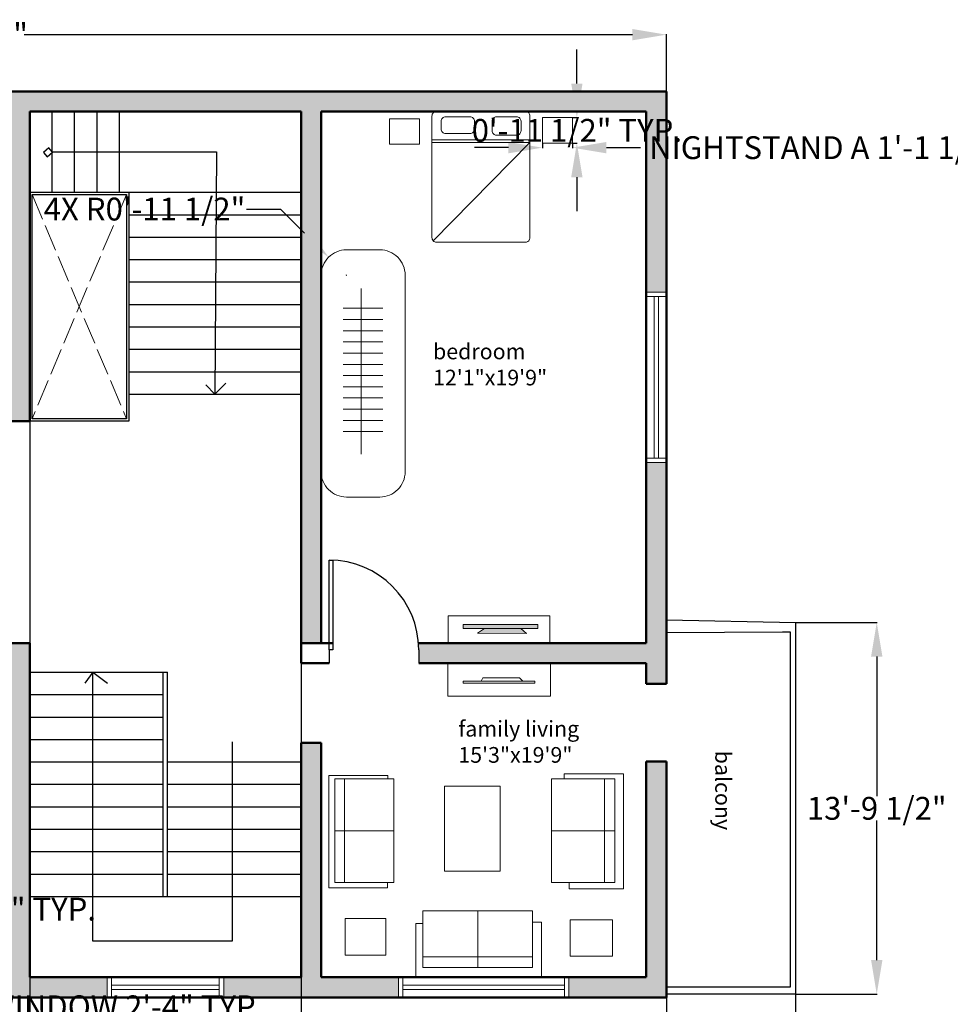
# Model space of a CAD drawing. Units: inches. Extents: x -2 to 7298, y -2 to 4583.
# Tile 5 of 6: x 6384 to 6799, y 4144 to 4583. Entities that reach past the tile are written whole.
import ezdxf

# ---------------------------------------------------------------- set-up
doc = ezdxf.new("R2010")
doc.units = ezdxf.units.IN
doc.header["$MEASUREMENT"] = 0
doc.linetypes.add('ACAD_ISO02W100', pattern=[15, 12, -3])
for name, color, linetype, lineweight in [('A-ANNO-DIMS', 2, 'Continuous', 18), ('A-AREA-IDEN', 7, 'Continuous', 18), ('A-DOOR', 4, 'Continuous', 25), ('A-FLOR-BALC', 7, 'Continuous', 25), ('A-FLOR-CASE', 30, 'Continuous', 18), ('A-FLOR-STRS', 7, 'Continuous', 25), ('A-FLOR-STRS-HIDN', 7, 'ACAD_ISO02W100', 18), ('A-FURN', 8, 'Continuous', 18), ('A-FURN-PATT', 18, 'Continuous', 13), ('A-GLAZ', 4, 'Continuous', 18), ('A-WALL', 7, 'Continuous', 50), ('A-WALL-PATT', 18, 'Continuous', 13)]:
    doc.layers.add(name, color=color, linetype=linetype, lineweight=lineweight)
doc.styles.get("Standard").update_dxf_attribs({"font": 'arial.ttf'})
doc.dimstyles.get("Standard").update_dxf_attribs({"dimtxt": 10.18, "dimasz": 15.18, "dimexe": 0.18, "dimexo": 0.0625, "dimgap": 0.09, "dimtad": 0, "dimtih": 1, "dimtoh": 1, "dimdec": 0, "dimzin": 0, "dimdsep": 46, "dimlunit": 3, "dimtxsty": 'Standard', "dimcen": 0.09, "dimadec": 0, "dimazin": 0, "dimtfac": 1, "dimtdec": 0, "dimtofl": 0, "dimtmove": 0, "dimatfit": 3, "dimfxl": 1, "dimtolj": 1, "dimtzin": 0, "dimarcsym": 0})

# ---------------------------------------------------------------- blocks, each defined once
blk = doc.blocks.new('*U2')
for p, q in [((0, 0), (0, -6)), ((40, 0), (40, -6))]:
    blk.add_line(p, q)
blk.add_lwpolyline([(0, 0), (0, 40), (1.75, 40), (1.75, 0)], close=True)
blk.add_arc((0, 0), 40, 0, 90)
blk = doc.blocks.new('*D5')
at = {"layer": 'A-ANNO-DIMS', "color": 0, "lineweight": -2, "transparency": 16777216}
for p, q in [((6064.27, 4551.54), (6064.27, 4576.93)), ((6079.45, 4576.75), (6350.69, 4576.75)), ((6657.09, 4576.75), (6385.84, 4576.75)), ((6672.27, 4551.54), (6672.27, 4576.93))]:
    blk.add_line(p, q, dxfattribs=at)
at = {"layer": 'A-ANNO-DIMS', "color": 0, "transparency": 16777216}
for points in [[(6079.45, 4579.28), (6079.45, 4574.22), (6064.27, 4576.75)], [(6657.09, 4579.28), (6657.09, 4574.22), (6672.27, 4576.75)]]:
    blk.add_solid(points, dxfattribs=at)
at = {"layer": 'Defpoints', "color": 0, "transparency": 16777216}
for p in [(6672.27, 4576.75), (6064.27, 4551.48), (6672.27, 4551.48)]:
    blk.add_point(p, dxfattribs=at)
at = {"layer": 'A-ANNO-DIMS', "color": 0, "transparency": 16777216, "insert": (6368.27, 4576.75), "char_height": 10.18, "attachment_point": 5}
blk.add_mtext('\\A1;50\'-8"', dxfattribs=at)
blk = doc.blocks.new('WINDOW-72IN')
for p, q in [((-2, 4.5), (-2, -4.5)), ((0, 4.5), (0, -4.5)), ((72, 4.5), (72, -4.5)), ((74, 4.5), (74, -4.5)), ((0, 1), (72, 1)), ((0, -1), (72, -1))]:
    blk.add_line(p, q)
blk = doc.blocks.new('WINDOW-48IN')
for p, q in [((-2, 4.5), (-2, -4.5)), ((0, 4.5), (0, -4.5)), ((48, 4.5), (48, -4.5)), ((50, 4.5), (50, -4.5)), ((0, 1), (48, 1)), ((0, -1), (48, -1))]:
    blk.add_line(p, q)
blk = doc.blocks.new('NIGHTSTAND-A')
blk.add_lwpolyline([(13.38, 11.39), (13.38, 11.39), (0, 11.39), (0, 11.39), (0, 0), (0, 0), (13.38, 0), (13.38, 0)], close=True)
blk = doc.blocks.new('*D39')
at = {"layer": 'A-ANNO-DIMS', "color": 0, "lineweight": -2, "transparency": 16777216}
for p, q in [((6308.27, 4147.41), (6308.27, 4143.1)), ((6336.27, 4147.41), (6336.27, 4143.1)), ((6293.09, 4143.28), (6277.91, 4143.28)), ((6351.45, 4143.28), (6366.63, 4143.28))]:
    blk.add_line(p, q, dxfattribs=at)
at = {"layer": 'A-ANNO-DIMS', "color": 0, "transparency": 16777216}
for points in [[(6293.09, 4145.81), (6293.09, 4140.75), (6308.27, 4143.28)], [(6351.45, 4145.81), (6351.45, 4140.75), (6336.27, 4143.28)]]:
    blk.add_solid(points, dxfattribs=at)
at = {"layer": 'Defpoints', "color": 0, "transparency": 16777216}
for p in [(6308.27, 4147.48), (6336.27, 4147.48), (6336.27, 4143.28)]:
    blk.add_point(p, dxfattribs=at)
at = {"layer": 'A-ANNO-DIMS', "color": 0, "transparency": 16777216, "insert": (6431.13, 4143.28), "char_height": 10.18, "attachment_point": 5}
blk.add_mtext('\\A1;WINDOW 2\'-4" TYP.', dxfattribs=at)
blk = doc.blocks.new('*D40')
at = {"layer": 'A-ANNO-DIMS', "color": 0, "lineweight": -2, "transparency": 16777216}
for p, q in [((6340.47, 4171.66), (6340.47, 4186.84)), ((6340.47, 4186.84), (6355.65, 4186.84)), ((6336.33, 4156.48), (6340.65, 4156.48)), ((6336.33, 4147.48), (6340.65, 4147.48)), ((6340.47, 4132.3), (6340.47, 4117.12))]:
    blk.add_line(p, q, dxfattribs=at)
at = {"layer": 'A-ANNO-DIMS', "color": 0, "transparency": 16777216}
for points in [[(6337.94, 4171.66), (6343, 4171.66), (6340.47, 4156.48)], [(6337.94, 4132.3), (6343, 4132.3), (6340.47, 4147.48)]]:
    blk.add_solid(points, dxfattribs=at)
at = {"layer": 'Defpoints', "color": 0, "transparency": 16777216}
for p in [(6336.27, 4156.48), (6340.47, 4156.48), (6336.27, 4147.48)]:
    blk.add_point(p, dxfattribs=at)
at = {"layer": 'A-ANNO-DIMS', "color": 0, "transparency": 16777216, "insert": (6386.76, 4186.84), "char_height": 10.18, "attachment_point": 5}
blk.add_mtext('\\A1;0\'-9" TYP.', dxfattribs=at)
blk = doc.blocks.new('*D53')
at = {"layer": 'A-ANNO-DIMS', "color": 0, "lineweight": -2, "transparency": 16777216}
for p, q in [((6616.96, 4528.32), (6616.96, 4526.19)), ((6630.33, 4528.32), (6630.33, 4526.19)), ((6601.78, 4526.37), (6586.6, 4526.37)), ((6645.51, 4526.37), (6660.69, 4526.37))]:
    blk.add_line(p, q, dxfattribs=at)
at = {"layer": 'A-ANNO-DIMS', "color": 0, "transparency": 16777216}
for points in [[(6601.78, 4528.9), (6601.78, 4523.84), (6616.96, 4526.37)], [(6645.51, 4528.9), (6645.51, 4523.84), (6630.33, 4526.37)]]:
    blk.add_solid(points, dxfattribs=at)
at = {"layer": 'Defpoints', "color": 0, "transparency": 16777216}
for p in [(6616.96, 4528.38), (6630.33, 4528.38), (6630.33, 4526.37)]:
    blk.add_point(p, dxfattribs=at)
at = {"layer": 'A-ANNO-DIMS', "color": 0, "transparency": 16777216, "insert": (6758.34, 4526.37), "char_height": 10.18, "attachment_point": 5}
blk.add_mtext('\\A1;NIGHTSTAND A 1\'-1 1/2" TYP.', dxfattribs=at)
blk = doc.blocks.new('*D54')
at = {"layer": 'A-ANNO-DIMS', "color": 0, "lineweight": -2, "transparency": 16777216}
for p, q in [((6632.34, 4554.95), (6632.34, 4570.13)), ((6630.4, 4539.77), (6632.52, 4539.77)), ((6630.4, 4528.38), (6632.52, 4528.38)), ((6632.34, 4513.2), (6632.34, 4498.02))]:
    blk.add_line(p, q, dxfattribs=at)
at = {"layer": 'A-ANNO-DIMS', "color": 0, "transparency": 16777216}
for points in [[(6629.81, 4554.95), (6634.87, 4554.95), (6632.34, 4539.77)], [(6629.81, 4513.2), (6634.87, 4513.2), (6632.34, 4528.38)]]:
    blk.add_solid(points, dxfattribs=at)
at = {"layer": 'Defpoints', "color": 0, "transparency": 16777216}
for p in [(6630.33, 4539.77), (6632.34, 4539.77), (6630.33, 4528.38)]:
    blk.add_point(p, dxfattribs=at)
at = {"layer": 'A-ANNO-DIMS', "color": 0, "transparency": 16777216, "insert": (6632.34, 4534.07), "char_height": 10.18, "attachment_point": 5}
blk.add_mtext('\\A1;0\'-11 1/2" TYP.', dxfattribs=at)
blk = doc.blocks.new('*D69')
at = {"layer": 'A-ANNO-DIMS', "color": 0, "lineweight": -2, "transparency": 16777216}
for p, q in [((6672.267047, 4147.414044), (6672.267047, 4060.046544)), ((6729.865325, 4148.84694), (6729.865325, 4060.046544)), ((6657.087047, 4060.226544), (6641.907047, 4060.226544)), ((6745.045325, 4060.226544), (6760.225325, 4060.226544))]:
    blk.add_line(p, q, dxfattribs=at)
at = {"layer": 'A-ANNO-DIMS', "color": 0, "transparency": 16777216}
for points in [[(6657.087047, 4062.756544), (6657.087047, 4057.696544), (6672.267047, 4060.226544)], [(6745.045325, 4062.756544), (6745.045325, 4057.696544), (6729.865325, 4060.226544)]]:
    blk.add_solid(points, dxfattribs=at)
at = {"layer": 'Defpoints', "color": 0, "transparency": 16777216}
for p in [(6672.267047, 4147.476544), (6729.865325, 4148.90944), (6729.865325, 4060.226544)]:
    blk.add_point(p, dxfattribs=at)
at = {"layer": 'A-ANNO-DIMS', "color": 0, "transparency": 16777216, "insert": (6701.066186, 4060.226544), "char_height": 10.18, "attachment_point": 5}
blk.add_mtext('\\A1;4\'-9 1/2"', dxfattribs=at)
blk = doc.blocks.new('*D70')
at = {"layer": 'A-ANNO-DIMS', "color": 0, "lineweight": -2, "transparency": 16777216}
for p, q in [((6729.93, 4314.65), (6766.3, 4314.65)), ((6766.12, 4299.47), (6766.12, 4237.14)), ((6766.12, 4164.09), (6766.12, 4226.42)), ((6729.93, 4148.91), (6766.3, 4148.91))]:
    blk.add_line(p, q, dxfattribs=at)
at = {"layer": 'A-ANNO-DIMS', "color": 0, "transparency": 16777216}
for points in [[(6763.59, 4299.47), (6768.65, 4299.47), (6766.12, 4314.65)], [(6763.59, 4164.09), (6768.65, 4164.09), (6766.12, 4148.91)]]:
    blk.add_solid(points, dxfattribs=at)
at = {"layer": 'Defpoints', "color": 0, "transparency": 16777216}
for p in [(6729.87, 4314.65), (6766.12, 4314.65), (6729.87, 4148.91)]:
    blk.add_point(p, dxfattribs=at)
at = {"layer": 'A-ANNO-DIMS', "color": 0, "transparency": 16777216, "insert": (6766.12, 4231.78), "char_height": 10.18, "attachment_point": 5}
blk.add_mtext('\\A1;13\'-9 1/2"', dxfattribs=at)
blk = doc.blocks.new('*D71')
at = {"layer": 'A-ANNO-DIMS', "color": 0, "lineweight": -2, "transparency": 16777216}
for p, q in [((6509.27, 4416.41), (6509.27, 4060.05)), ((6388.27, 4404.41), (6388.27, 4060.05)), ((6403.45, 4060.23), (6431.67, 4060.23)), ((6494.09, 4060.23), (6465.86, 4060.23))]:
    blk.add_line(p, q, dxfattribs=at)
at = {"layer": 'A-ANNO-DIMS', "color": 0, "transparency": 16777216}
for points in [[(6403.45, 4062.76), (6403.45, 4057.7), (6388.27, 4060.23)], [(6494.09, 4062.76), (6494.09, 4057.7), (6509.27, 4060.23)]]:
    blk.add_solid(points, dxfattribs=at)
at = {"layer": 'Defpoints', "color": 0, "transparency": 16777216}
for p in [(6509.27, 4416.48), (6388.27, 4404.48), (6509.27, 4060.23)]:
    blk.add_point(p, dxfattribs=at)
at = {"layer": 'A-ANNO-DIMS', "color": 0, "transparency": 16777216, "insert": (6448.77, 4060.23), "char_height": 10.18, "attachment_point": 5}
blk.add_mtext('\\A1;10\'-1"', dxfattribs=at)
blk = doc.blocks.new('*D95')
at = {"layer": 'A-ANNO-DIMS', "color": 0, "lineweight": -2, "transparency": 16777216}
for p, q in [((6484.92, 4498.99), (6500.1, 4498.99)), ((6500.1, 4498.99), (6510.83, 4488.26)), ((6529.44, 4469.56), (6529.62, 4469.56)), ((6529.53, 4469.47), (6529.53, 4469.65))]:
    blk.add_line(p, q, dxfattribs=at)
at = {"layer": 'A-ANNO-DIMS', "color": 0, "transparency": 16777216}
blk.add_solid([(6512.62, 4490.05), (6509.04, 4486.47), (6521.57, 4477.53)], dxfattribs=at)
at = {"layer": 'Defpoints', "color": 0, "transparency": 16777216}
for p in [(6521.57, 4477.53), (6529.53, 4469.56)]:
    blk.add_point(p, dxfattribs=at)
at = {"layer": 'A-ANNO-DIMS', "color": 0, "transparency": 16777216, "insert": (6439.47, 4498.99), "char_height": 10.18, "attachment_point": 5}
blk.add_mtext('\\A1;4X R0\'-11 1/2"', dxfattribs=at)

msp = doc.modelspace()

# ---------------------------------------------------------------- hatches: boundary and pattern name
at = {"layer": 'A-FURN-PATT'}
h = msp.add_hatch(color=256, dxfattribs=at)
h.dxf.hatch_style = 1
h.paths.add_polyline_path([(6607.35, 4311.96), (6591.2, 4311.96), (6588, 4309.84), (6609.92, 4309.8)])
h.paths.add_polyline_path([(6614.99, 4313.76), (6581.62, 4313.76), (6581.62, 4311.96), (6614.99, 4311.96)])
at = {"layer": 'A-WALL-PATT'}
h = msp.add_hatch(color=256, dxfattribs=at)
h.dxf.hatch_style = 1
h.paths.add_polyline_path([(6073.27, 4434.19), (6064.27, 4434.19), (6064.27, 4303.39), (6073.27, 4303.39), (6073.27, 4305.48)])
h.paths.add_polyline_path([(6265.27, 4348.36), (6256.27, 4348.36), (6256.27, 4345.36), (6073.27, 4345.36), (6073.27, 4336.36), (6256.27, 4336.36), (6256.27, 4331.36), (6260.77, 4331.36), (6260.77, 4333.36), (6265.27, 4333.36)])
h.paths.add_polyline_path([(6073.27, 4251.39), (6064.27, 4251.39), (6064.27, 4147.48), (6308.27, 4147.48), (6308.27, 4156.48), (6265.27, 4156.48), (6265.27, 4256.48), (6265.27, 4261.07), (6340.27, 4261.07), (6340.27, 4263.57, -0.014283), (6340.27, 4265.57), (6340.27, 4270.07), (6265.27, 4270.07), (6265.27, 4297.36), (6261.6, 4297.36, -0.036646), (6256.27, 4297.69), (6256.27, 4156.48), (6073.27, 4156.48)])
h.paths.add_polyline_path([(6422.77, 4156.48), (6388.27, 4156.48), (6388.27, 4305.48), (6379.27, 4305.48), (6379.27, 4270.07), (6379.27, 4261.07), (6379.27, 4156.48), (6336.27, 4156.48), (6336.27, 4147.48), (6422.77, 4147.48)])
h.paths.add_polyline_path([(6552.77, 4156.48), (6518.27, 4156.48), (6518.27, 4261.05), (6509.27, 4261.05), (6509.27, 4156.48), (6474.77, 4156.48), (6474.77, 4147.48), (6552.77, 4147.48)])
h.paths.add_polyline_path([(6672.27, 4252.66), (6663.27, 4252.66), (6663.27, 4156.48), (6628.77, 4156.48), (6628.77, 4147.48), (6672.27, 4147.48)])
h.paths.add_polyline_path([(6672.27, 4385.98), (6663.27, 4385.98), (6663.27, 4305.48), (6561.68, 4305.48, -0.01877), (6561.79, 4302.48), (6561.79, 4296.48), (6663.27, 4296.48), (6663.27, 4287.22), (6672.27, 4287.22)])
h.paths.add_polyline_path([(6518.27, 4542.48), (6663.27, 4542.48), (6663.27, 4461.98), (6672.27, 4461.98), (6672.27, 4551.48), (6336.27, 4551.48), (6336.27, 4542.48), (6379.27, 4542.48), (6379.27, 4404.48), (6388.27, 4404.48), (6388.27, 4506.48), (6388.27, 4542.48), (6509.27, 4542.48), (6509.27, 4413.48), (6509.27, 4404.48), (6509.27, 4305.48), (6518.27, 4305.48)])
h.paths.add_polyline_path([(6379.27, 4422.48), (6319.12, 4422.48), (6319.12, 4419.98, -0.014283), (6319.12, 4417.98), (6319.12, 4413.48), (6379.27, 4413.48)])
h.paths.add_polyline_path([(6265.27, 4542.48), (6308.27, 4542.48), (6308.27, 4551.48), (6221.92, 4551.48), (6221.92, 4542.48), (6256.27, 4542.48), (6256.27, 4384.36), (6258.77, 4384.36, -0.014283), (6260.77, 4384.36), (6265.27, 4384.36)])
h.paths.add_polyline_path([(6169.92, 4551.48), (6064.27, 4551.48), (6064.27, 4486.19), (6073.27, 4486.19), (6073.27, 4542.48), (6169.92, 4542.48)])

# ---------------------------------------------------------------- linework, layer by layer
at = {"layer": 'A-FLOR-BALC'}
for p, q in [((6672.27, 4315.87), (6672.27, 4315.87)), ((6672.27, 4315.87), (6729.87, 4314.65)), ((6729.87, 4314.65), (6729.87, 4148.91)), ((6672.27, 4310.16), (6724.01, 4310.55)), ((6672.27, 4310.16), (6672.27, 4310.16)), ((6724.01, 4310.55), (6727.45, 4310.55)), ((6727.45, 4310.55), (6727.45, 4152.03)), ((6727.45, 4152.03), (6672.27, 4152.03)), ((6729.87, 4148.91), (6672.27, 4148.91))]:
    msp.add_line(p, q, dxfattribs=at)
at = {"layer": 'A-FLOR-CASE'}
for p, q in [((6536.09, 4463.61), (6536.09, 4389.67)), ((6528.11, 4454.75), (6545.84, 4454.75)), ((6528.11, 4449.75), (6545.84, 4449.75)), ((6528.11, 4444.75), (6545.84, 4444.75)), ((6528.11, 4439.75), (6545.84, 4439.75)), ((6528.11, 4434.75), (6545.84, 4434.75)), ((6528.11, 4429.75), (6545.84, 4429.75)), ((6528.11, 4424.75), (6545.84, 4424.75)), ((6528.11, 4419.75), (6545.84, 4419.75)), ((6528.11, 4414.75), (6545.84, 4414.75)), ((6528.11, 4409.75), (6545.84, 4409.75)), ((6528.11, 4404.75), (6545.84, 4404.75)), ((6528.11, 4404.75), (6545.84, 4404.75)), ((6528.11, 4399.75), (6545.84, 4399.75))]:
    msp.add_line(p, q, dxfattribs=at)
msp.add_lwpolyline([(6518.27, 4469.56, -0.414214), (6529.53, 4480.83), (6544.46, 4480.83, -0.414214), (6555.73, 4469.56), (6555.73, 4381.86, -0.414214), (6544.46, 4370.59), (6529.53, 4370.59, -0.414214), (6518.27, 4381.86)], format="xyb", close=True, dxfattribs=at)
at = {"layer": 'A-FLOR-STRS'}
for p, q in [((6398.27, 4506.48), (6398.27, 4542.48)), ((6408.27, 4506.48), (6408.27, 4542.48)), ((6418.27, 4506.48), (6418.27, 4542.48)), ((6428.27, 4506.48), (6428.27, 4542.48)), ((6396.77, 4526.26), (6394.33, 4524.22)), ((6394.33, 4524.22), (6395.99, 4522.24)), ((6395.99, 4522.24), (6398.43, 4524.29)), ((6398.27, 4524.48), (6396.77, 4526.26)), ((6398.27, 4524.48), (6471.6, 4524.48)), ((6471.6, 4524.48), (6470.84, 4416.48)), ((6432.41, 4506.48), (6509.27, 4506.48)), ((6432.41, 4496.48), (6509.27, 4496.48)), ((6432.41, 4486.48), (6509.27, 4486.48)), ((6432.41, 4476.48), (6509.27, 4476.48)), ((6432.41, 4466.48), (6509.27, 4466.48)), ((6432.41, 4456.48), (6509.27, 4456.48)), ((6432.41, 4446.48), (6509.27, 4446.48)), ((6432.41, 4436.48), (6509.27, 4436.48)), ((6432.41, 4426.48), (6509.27, 4426.48)), ((6470.84, 4416.48), (6475.72, 4421.33)), ((6470.84, 4416.48), (6466.74, 4420.6)), ((6432.41, 4416.48), (6509.27, 4416.48)), ((6388.27, 4292.48), (6449.77, 4292.48)), ((6416.47, 4292.48), (6412.8, 4287.64)), ((6416.47, 4172.5), (6416.47, 4292.48)), ((6416.47, 4292.48), (6422.93, 4287.57)), ((6447.77, 4192.48), (6447.77, 4292.48)), ((6449.77, 4192.48), (6449.77, 4292.48)), ((6388.27, 4282.48), (6447.77, 4282.48)), ((6388.27, 4272.48), (6447.77, 4272.48)), ((6388.27, 4262.48), (6447.77, 4262.48)), ((6478.57, 4261.41), (6478.57, 4172.5)), ((6388.27, 4252.48), (6447.77, 4252.48)), ((6449.77, 4252.48), (6509.27, 4252.48)), ((6388.27, 4242.48), (6447.77, 4242.48)), ((6449.77, 4242.48), (6509.27, 4242.48)), ((6388.27, 4232.48), (6447.77, 4232.48)), ((6449.77, 4232.48), (6509.27, 4232.48)), ((6388.27, 4222.48), (6447.77, 4222.48)), ((6449.77, 4222.48), (6509.27, 4222.48)), ((6388.27, 4212.48), (6447.77, 4212.48)), ((6449.77, 4212.48), (6509.27, 4212.48)), ((6388.27, 4202.48), (6447.77, 4202.48)), ((6449.77, 4202.48), (6509.27, 4202.48)), ((6388.27, 4192.48), (6509.27, 4192.48)), ((6478.57, 4172.5), (6416.47, 4172.5))]:
    msp.add_line(p, q, dxfattribs=at)
for points in [[(6388.27, 4506.48), (6388.27, 4506.48), (6432.41, 4506.48), (6432.41, 4506.48), (6432.41, 4404.48), (6432.41, 4404.48), (6388.27, 4404.48), (6388.27, 4404.48)], [(6389.27, 4505.48), (6431.41, 4505.48), (6431.41, 4405.48), (6389.27, 4405.48)]]:
    msp.add_lwpolyline(points, close=True, dxfattribs=at)
at = {"layer": 'A-FLOR-STRS-HIDN'}
for p, q in [((6389.27, 4505.48), (6431.41, 4405.48)), ((6431.41, 4505.48), (6389.27, 4405.48))]:
    msp.add_line(p, q, dxfattribs=at)
at = {"layer": 'A-FURN'}
for p, q in [((6567.68, 4529.79), (6611.43, 4529.79)), ((6567.68, 4528.64), (6611.43, 4528.64)), ((6568.27, 4484.84), (6611.43, 4528.64)), ((6588, 4309.84), (6591.2, 4311.96)), ((6609.92, 4309.8), (6607.35, 4311.96)), ((6588, 4309.84), (6609.92, 4309.8)), ((6589.69, 4288.43), (6590.38, 4290.03)), ((6590.38, 4290.03), (6606.72, 4290.03)), ((6606.72, 4290.03), (6608.22, 4288.43)), ((6521.64, 4246.35), (6521.64, 4196.37)), ((6521.64, 4246.35), (6547.97, 4246.35)), ((6547.97, 4244.86), (6547.97, 4246.35)), ((6626.63, 4247.23), (6626.63, 4244.86)), ((6653.16, 4247.23), (6626.63, 4247.23)), ((6653.16, 4195.87), (6653.16, 4247.23)), ((6528.65, 4244.86), (6528.65, 4198.67)), ((6644.67, 4244.86), (6644.67, 4198.67)), ((6524.38, 4221.76), (6550.75, 4221.76)), ((6621.08, 4221.76), (6649.3, 4221.76)), ((6547.89, 4196.37), (6547.89, 4198.67)), ((6628.94, 4198.67), (6628.94, 4195.87)), ((6521.64, 4196.37), (6547.89, 4196.37)), ((6628.94, 4195.87), (6653.16, 4195.87)), ((6588.11, 4160.76), (6588.11, 4186.13)), ((6563.65, 4180.41), (6560.51, 4180.41)), ((6560.51, 4180.41), (6560.51, 4156.48)), ((6616.56, 4180.99), (6612.56, 4180.99)), ((6616.56, 4156.48), (6616.56, 4180.99)), ((6563.65, 4165.56), (6612.56, 4165.56)), ((6560.51, 4156.48), (6616.56, 4156.48))]:
    msp.add_line(p, q, dxfattribs=at)
for points in [[(6611.43, 4540.48, 0.414214), (6609.43, 4542.48), (6569.68, 4542.48, 0.414214), (6567.68, 4540.48), (6567.68, 4486.26, 0.414214), (6569.68, 4484.26), (6609.43, 4484.26, 0.414214), (6611.43, 4486.26)], [(6571.77, 4538.1, -0.414214), (6573.77, 4540.1), (6584.66, 4540.1, -0.414214), (6586.66, 4538.1), (6586.66, 4534.67, -0.414214), (6584.66, 4532.67), (6573.77, 4532.67, -0.414214), (6571.77, 4534.67)], [(6594.49, 4538.17, -0.414214), (6596.49, 4540.17), (6605.42, 4540.17, -0.414214), (6607.42, 4538.17), (6607.42, 4533.92, -0.414214), (6605.42, 4531.92), (6596.49, 4531.92, -0.414214), (6594.49, 4533.92)]]:
    msp.add_lwpolyline(points, format="xyb", close=True, dxfattribs=at)
for points in [[(6574.91, 4305.48), (6574.91, 4305.48), (6620.23, 4305.48), (6620.23, 4305.48), (6620.23, 4317.68), (6620.23, 4317.68), (6574.91, 4317.68), (6574.91, 4317.68)], [(6581.62, 4313.76), (6581.62, 4313.76), (6614.99, 4313.76), (6614.99, 4313.76), (6614.99, 4311.96), (6614.99, 4311.96), (6581.62, 4311.96), (6581.62, 4311.96)], [(6574.71, 4296.48), (6620.56, 4296.48), (6620.56, 4281.82), (6574.71, 4281.82)], [(6581.62, 4288.43), (6613.6, 4288.43), (6613.6, 4287.54), (6581.62, 4287.54)], [(6550.75, 4244.86), (6524.38, 4244.86), (6524.38, 4198.67), (6550.75, 4198.67)], [(6573.25, 4241.67), (6598.12, 4241.67), (6598.12, 4203.81), (6573.25, 4203.81)], [(6621.08, 4244.86), (6649.3, 4244.86), (6649.3, 4198.67), (6621.08, 4198.67)], [(6563.65, 4186.13), (6612.56, 4186.13), (6612.56, 4160.76), (6563.65, 4160.76)], [(6528.98, 4182.62), (6547.1, 4182.62), (6547.1, 4166.24), (6528.98, 4166.24)], [(6629.41, 4182.01), (6648.22, 4182.01), (6648.22, 4165.83), (6629.41, 4165.83)]]:
    msp.add_lwpolyline(points, close=True, dxfattribs=at)
at = {"layer": 'A-GLAZ'}
msp.add_line((6663.27, 4423.98), (6663.27, 4423.98), dxfattribs=at)
at = {"layer": 'A-WALL'}
for p, q in [((6672.27, 4551.48), (6064.27, 4551.48)), ((6672.27, 4287.22), (6672.27, 4551.48)), ((6509.27, 4542.48), (6388.27, 4542.48)), ((6388.27, 4404.48), (6388.27, 4542.48)), ((6509.27, 4413.48), (6509.27, 4542.48)), ((6663.27, 4542.48), (6518.27, 4542.48)), ((6518.27, 4305.48), (6518.27, 4542.48)), ((6663.27, 4305.48), (6663.27, 4542.48)), ((6509.27, 4413.48), (6509.27, 4404.48)), ((6379.27, 4404.48), (6388.27, 4404.48)), ((6509.27, 4296.48), (6509.27, 4404.48)), ((6388.27, 4305.48), (6379.27, 4305.48)), ((6388.27, 4156.48), (6388.27, 4305.48)), ((6523.54, 4305.48), (6509.27, 4305.48)), ((6663.27, 4305.48), (6561.68, 4305.48)), ((6521.79, 4296.48), (6509.27, 4296.48)), ((6663.27, 4296.48), (6561.79, 4296.48)), ((6663.27, 4287.22), (6663.27, 4296.48)), ((6663.27, 4287.22), (6672.27, 4287.22)), ((6509.27, 4156.48), (6509.27, 4261.05)), ((6509.27, 4261.05), (6518.27, 4261.05)), ((6518.27, 4156.48), (6518.27, 4261.05)), ((6663.27, 4156.48), (6663.27, 4252.66)), ((6663.27, 4252.66), (6672.27, 4252.66)), ((6672.27, 4147.48), (6672.27, 4252.66)), ((6388.27, 4156.48), (6509.27, 4156.48)), ((6518.27, 4156.48), (6663.27, 4156.48)), ((6064.27, 4147.48), (6672.27, 4147.48))]:
    msp.add_line(p, q, dxfattribs=at)

# ---------------------------------------------------------------- block references
at = {"layer": 'A-DOOR'}
msp.add_blockref('*U2', (6521.79, 4302.48), dxfattribs=at)
at = {"layer": 'A-FURN'}
for p in [(6616.96, 4528.38), (6548.73, 4527.87)]:
    msp.add_blockref('NIGHTSTAND-A', p, dxfattribs=at)
at = {"layer": 'A-GLAZ', "rotation": 89.9999999999985}
msp.add_blockref('WINDOW-72IN', (6667.77, 4387.98), dxfattribs=at)
at = {"layer": 'A-GLAZ'}
for name, p in [('WINDOW-48IN', (6424.77, 4151.98)), ('WINDOW-72IN', (6554.77, 4151.98))]:
    msp.add_blockref(name, p, dxfattribs=at)

# ---------------------------------------------------------------- texts
at = {"layer": 'A-AREA-IDEN', "char_height": 7, "attachment_point": 1}
for s, insert in [('bedroom\\P12\'1"x19\'9"', (6568.17, 4439.01)), ('family living\\P15\'3"x19\'9"', (6579.46, 4270.77))]:
    msp.add_mtext_dynamic_manual_height_columns(s, width=119.0967, gutter_width=1, heights=[0], dxfattribs=dict(at, insert=insert))
at = {"layer": 'A-AREA-IDEN', "insert": (6701.07, 4257.51), "char_height": 7, "attachment_point": 1, "rotation": 270}
msp.add_mtext_dynamic_manual_height_columns('balcony', width=12.4828, gutter_width=1, heights=[0], dxfattribs=at)

# ---------------------------------------------------------------- dimensions: what is measured, and where the dimension line sits
at = {"layer": 'A-ANNO-DIMS'}
for base, p1, p2, override, picture, middle in [((6672.27, 4576.75), (6064.27, 4551.48), (6672.27, 4551.48), {"dimclrd": 0, "dimclre": 0, "dimclrt": 0}, '*D5', (6368.27, 4576.75)), ((6509.27, 4060.23), (6388.27, 4404.48), (6509.27, 4416.48), {"dimdec": 1, "dimlfac": 1, "dimrnd": 0, "dimzin": 1, "dimdsep": 46, "dimlunit": 4, "dimfrac": 2}, '*D71', (6448.77, 4060.23)), ((6729.87, 4060.23), (6672.27, 4147.48), (6729.87, 4148.91), {"dimdec": 1, "dimlfac": 1, "dimrnd": 0, "dimzin": 1, "dimdsep": 46, "dimlunit": 4, "dimfrac": 2}, '*D69', (6701.07, 4060.23))]:
    dim = msp.add_linear_dim(base=base, p1=p1, p2=p2, dimstyle='Standard', override=override, dxfattribs=at)
    dim.commit()
    dim.dimension.update_dxf_attribs({"geometry": picture, "text_midpoint": middle})
for base, p1, p2, picture, middle in [((6632.34, 4539.77), (6630.33, 4528.38), (6630.33, 4539.77), '*D54', (6632.34, 4534.07)), ((6340.47, 4156.48), (6336.27, 4147.48), (6336.27, 4156.48), '*D40', (6386.76, 4186.84))]:
    dim = msp.add_linear_dim(base=base, p1=p1, p2=p2, angle=90, text='<> TYP.', dimstyle='Standard', override={"dimdec": 1, "dimlfac": 1, "dimrnd": 0, "dimzin": 1, "dimdsep": 46, "dimlunit": 4, "dimfrac": 2}, dxfattribs=at)
    dim.commit()
    dim.dimension.update_dxf_attribs({"geometry": picture, "text_midpoint": middle})
for base, p1, p2, text, picture, middle in [((6630.33, 4526.37), (6616.96, 4528.38), (6630.33, 4528.38), 'NIGHTSTAND A <> TYP.', '*D53', (6758.34, 4526.37)), ((6336.27, 4143.28), (6308.27, 4147.48), (6336.27, 4147.48), 'WINDOW <> TYP.', '*D39', (6431.13, 4143.28))]:
    dim = msp.add_linear_dim(base=base, p1=p1, p2=p2, text=text, dimstyle='Standard', override={"dimdec": 1, "dimlfac": 1, "dimrnd": 0, "dimzin": 1, "dimdsep": 46, "dimlunit": 4, "dimfrac": 2}, dxfattribs=at)
    dim.commit()
    dim.dimension.update_dxf_attribs({"geometry": picture, "text_midpoint": middle})
dim = msp.add_radius_dim(center=(6529.53, 4469.56), mpoint=(6521.57, 4477.53), text='4X <>', dimstyle='Standard', override={"dimdec": 1, "dimlfac": 1, "dimrnd": 0, "dimzin": 1, "dimdsep": 46, "dimlunit": 4, "dimfrac": 2}, dxfattribs=at)
dim.commit()
dim.dimension.update_dxf_attribs({"geometry": '*D95', "text_midpoint": (6439.47, 4498.99)})
dim = msp.add_linear_dim(base=(6766.12, 4314.65), p1=(6729.87, 4148.91), p2=(6729.87, 4314.65), angle=90, dimstyle='Standard', override={"dimdec": 1, "dimlfac": 1, "dimrnd": 0, "dimzin": 1, "dimdsep": 46, "dimlunit": 4, "dimfrac": 2}, dxfattribs=at)
dim.commit()
dim.dimension.update_dxf_attribs({"geometry": '*D70', "text_midpoint": (6766.12, 4231.78)})

doc.saveas('drawing.dxf')
